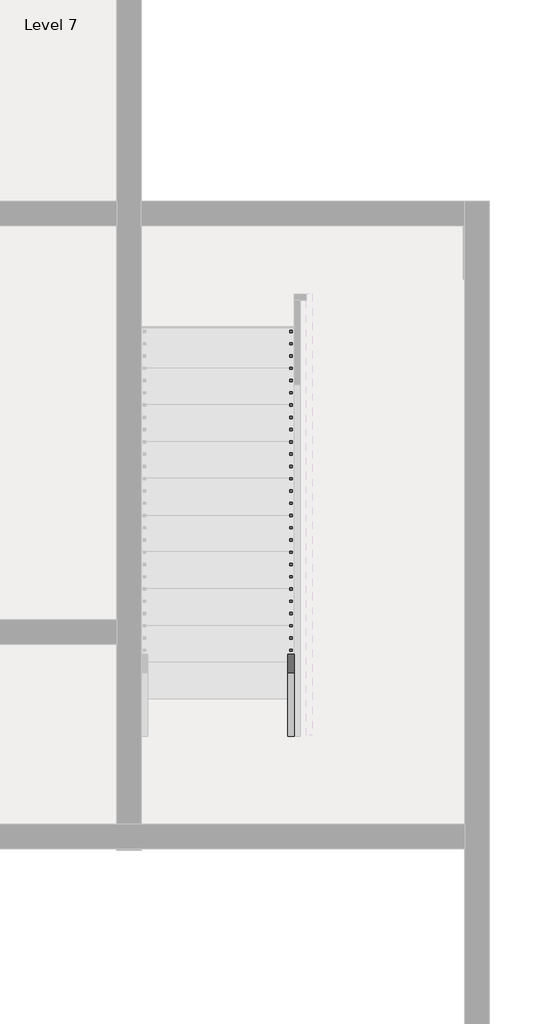
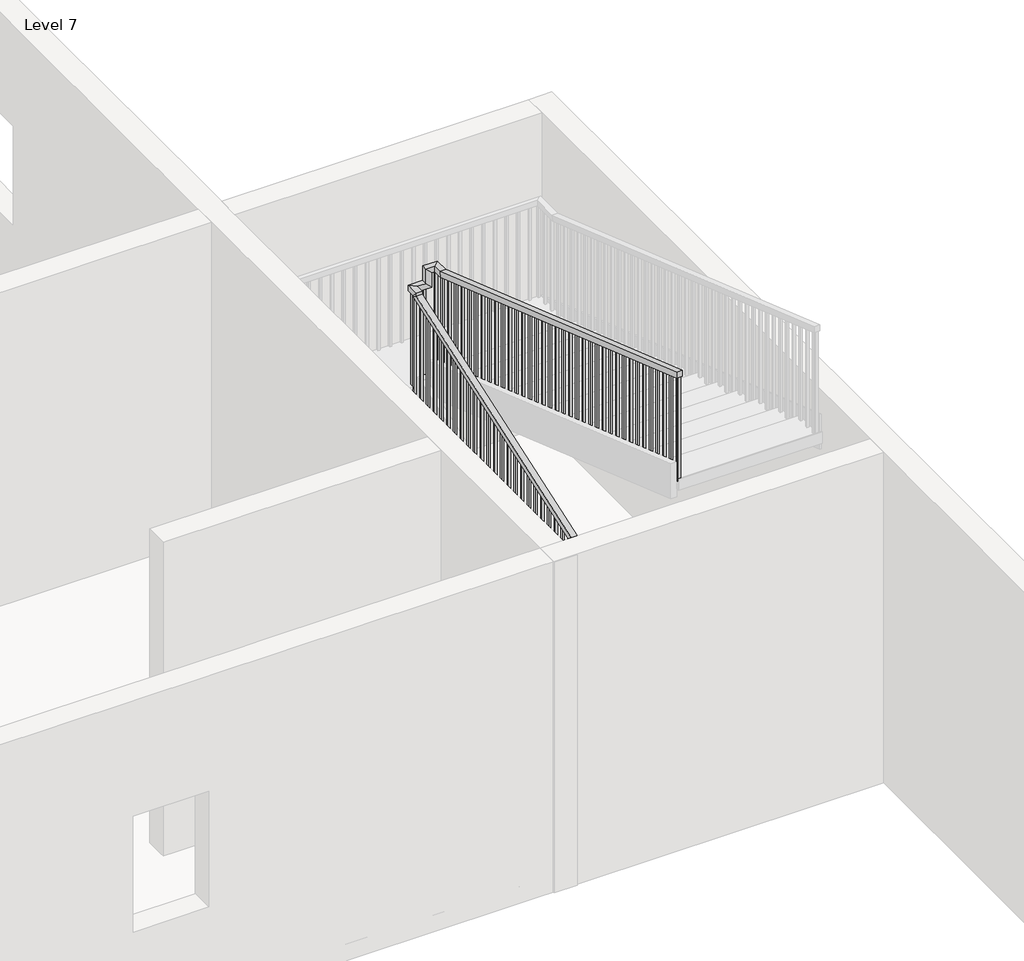
# One storey, part 6 of 14: 1 railing.
"""IFC4 building model written with IfcOpenShell, lengths in millimetres."""

from ifc_helpers import new_model, si_unit, frame, origin, place, context, project, spatial, polyline, outline, extrude, faceted_brep, element, save

model = new_model("IFC4")

# Units and contexts
model_context = context("Model", 3, world=origin())
ifc_project = project(units=[si_unit("LENGTHUNIT", "METRE", prefix="MILLI")], contexts=[model_context])

# Site, building, storey
site = spatial("IfcSite", under=ifc_project)
building = spatial("IfcBuilding", under=site)
storey = spatial("IfcBuildingStorey", under=building, Name="Level 7", Elevation=18288.0)

# Railing
placement = place(None, origin())
element("IfcRailing", 1, ObjectType="Handrail - Rectangular", at=placement, inside=storey, context=model_context, shape_type="SolidModel", body=[
    faceted_brep([(-2644.5381751, -9955.5916506, 19307.9076923), (-2644.5381751, -9955.5916506, 19254.1602476), (-2593.7381751, -9955.5916506, 19254.1602476), (-2593.7381751, -9955.5916506, 19307.9076923), (-2644.5381751, -6367.8416506, 20547.6687908), (-2644.5381751, -6317.0416506, 20511.4754856), (-2593.7381751, -6317.0416506, 20511.4754856), (-2593.7381751, -6367.8416506, 20547.6687908), (-2644.5381751, -6367.8416506, 20574.0), (-2644.5381751, -6317.0416506, 20523.2), (-2593.7381751, -6317.0416506, 20523.2), (-2593.7381751, -6367.8416506, 20574.0), (-2644.5381751, -6240.8416506, 20574.0), (-2644.5381751, -6240.8416506, 20523.2), (-2593.7381751, -6291.6416506, 20523.2), (-2593.7381751, -6291.6416506, 20574.0), (-2517.5381751, -6240.8416506, 20574.0), (-2466.7381751, -6240.8416506, 20523.2), (-2466.7381751, -6291.6416506, 20523.2), (-2517.5381751, -6291.6416506, 20574.0), (-2517.5381751, -6240.8416506, 20705.8846154), (-2466.7381751, -6240.8416506, 20655.0846154), (-2466.7381751, -6291.6416506, 20655.0846154), (-2517.5381751, -6291.6416506, 20705.8846154), (-2390.5381751, -6240.8416506, 20705.8846154), (-2390.5381751, -6240.8416506, 20655.0846154), (-2441.3381751, -6291.6416506, 20655.0846154), (-2441.3381751, -6291.6416506, 20705.8846154), (-2390.5381751, -6367.8416506, 20705.8846154), (-2390.5381751, -6376.3852679, 20655.0846154), (-2441.3381751, -6376.3852679, 20655.0846154), (-2441.3381751, -6367.8416506, 20705.8846154), (-2390.5381751, -9949.2416506, 21945.6), (-2441.3381751, -9949.2416506, 21945.6), (-2441.3381751, -9949.2416506, 21891.842594), (-2390.5381751, -9949.2416506, 21891.842594)], [[[0, 1, 2, 3]], [[1, 0, 4, 5]], [[2, 1, 5, 6]], [[3, 2, 6, 7]], [[0, 3, 7, 4]], [[5, 4, 8, 9]], [[6, 5, 9, 10]], [[7, 6, 10, 11]], [[4, 7, 11, 8]], [[9, 8, 12, 13]], [[10, 9, 13, 14]], [[11, 10, 14, 15]], [[8, 11, 15, 12]], [[13, 12, 16, 17]], [[14, 13, 17, 18]], [[15, 14, 18, 19]], [[12, 15, 19, 16]], [[17, 16, 20, 21]], [[18, 17, 21, 22]], [[19, 18, 22, 23]], [[16, 19, 23, 20]], [[21, 20, 24, 25]], [[22, 21, 25, 26]], [[23, 22, 26, 27]], [[20, 23, 27, 24]], [[25, 24, 28, 29]], [[26, 25, 29, 30]], [[27, 26, 30, 31]], [[24, 27, 31, 28]], [[32, 33, 34, 35]], [[29, 28, 32, 35]], [[30, 29, 35, 34]], [[31, 30, 34, 33]], [[28, 31, 33, 32]]]),
    extrude(outline(polyline([(-9933.3666506, 21886.3474017), (-9914.3166506, 21879.7531709), (-9914.3166506, 20925.6923077), (-9933.3666506, 20925.6923077), (-9933.3666506, 21886.3474017)])), frame((-2425.4631751, 0.0, 0.0), z_axis=(1.0, 0.0, 0.0), x_axis=(0.0, 1.0, 0.0)), (0.0, 0.0, 1.0), 19.05),
    extrude(outline(polyline([(-9831.7666506, 21851.1781709), (-9812.7166506, 21844.5839402), (-9812.7166506, 20925.6923077), (-9831.7666506, 20925.6923077), (-9831.7666506, 21851.1781709)])), frame((-2425.4631751, 0.0, 0.0), z_axis=(1.0, 0.0, 0.0), x_axis=(0.0, 1.0, 0.0)), (0.0, 0.0, 1.0), 19.05),
    extrude(outline(polyline([(-9730.1666506, 21816.0089402), (-9711.1166506, 21809.4147094), (-9711.1166506, 20925.6923077), (-9730.1666506, 20925.6923077), (-9730.1666506, 21816.0089402)])), frame((-2425.4631751, 0.0, 0.0), z_axis=(1.0, 0.0, 0.0), x_axis=(0.0, 1.0, 0.0)), (0.0, 0.0, 1.0), 19.05),
    extrude(outline(polyline([(-9628.5666506, 21780.8397094), (-9609.5166506, 21774.2454786), (-9609.5166506, 20820.1846154), (-9628.5666506, 20820.1846154), (-9628.5666506, 21780.8397094)])), frame((-2425.4631751, 0.0, 0.0), z_axis=(1.0, 0.0, 0.0), x_axis=(0.0, 1.0, 0.0)), (0.0, 0.0, 1.0), 19.05),
    extrude(outline(polyline([(-9526.9666506, 21745.6704786), (-9507.9166506, 21739.0762479), (-9507.9166506, 20820.1846154), (-9526.9666506, 20820.1846154), (-9526.9666506, 21745.6704786)])), frame((-2425.4631751, 0.0, 0.0), z_axis=(1.0, 0.0, 0.0), x_axis=(0.0, 1.0, 0.0)), (0.0, 0.0, 1.0), 19.05),
    extrude(outline(polyline([(-9425.3666506, 21710.5012479), (-9406.3166506, 21703.9070171), (-9406.3166506, 20820.1846154), (-9425.3666506, 20820.1846154), (-9425.3666506, 21710.5012479)])), frame((-2425.4631751, 0.0, 0.0), z_axis=(1.0, 0.0, 0.0), x_axis=(0.0, 1.0, 0.0)), (0.0, 0.0, 1.0), 19.05),
    extrude(outline(polyline([(-9323.7666506, 21675.3320171), (-9304.7166506, 21668.7377863), (-9304.7166506, 20714.6769231), (-9323.7666506, 20714.6769231), (-9323.7666506, 21675.3320171)])), frame((-2425.4631751, 0.0, 0.0), z_axis=(1.0, 0.0, 0.0), x_axis=(0.0, 1.0, 0.0)), (0.0, 0.0, 1.0), 19.05),
    extrude(outline(polyline([(-9222.1666506, 21640.1627863), (-9203.1166506, 21633.5685556), (-9203.1166506, 20714.6769231), (-9222.1666506, 20714.6769231), (-9222.1666506, 21640.1627863)])), frame((-2425.4631751, 0.0, 0.0), z_axis=(1.0, 0.0, 0.0), x_axis=(0.0, 1.0, 0.0)), (0.0, 0.0, 1.0), 19.05),
    extrude(outline(polyline([(-9120.5666506, 21604.9935556), (-9101.5166506, 21598.3993248), (-9101.5166506, 20714.6769231), (-9120.5666506, 20714.6769231), (-9120.5666506, 21604.9935556)])), frame((-2425.4631751, 0.0, 0.0), z_axis=(1.0, 0.0, 0.0), x_axis=(0.0, 1.0, 0.0)), (0.0, 0.0, 1.0), 19.05),
    extrude(outline(polyline([(-9018.9666506, 21569.8243248), (-8999.9166506, 21563.230094), (-8999.9166506, 20609.1692308), (-9018.9666506, 20609.1692308), (-9018.9666506, 21569.8243248)])), frame((-2425.4631751, 0.0, 0.0), z_axis=(1.0, 0.0, 0.0), x_axis=(0.0, 1.0, 0.0)), (0.0, 0.0, 1.0), 19.05),
    extrude(outline(polyline([(-8917.3666506, 21534.655094), (-8898.3166506, 21528.0608632), (-8898.3166506, 20609.1692308), (-8917.3666506, 20609.1692308), (-8917.3666506, 21534.655094)])), frame((-2425.4631751, 0.0, 0.0), z_axis=(1.0, 0.0, 0.0), x_axis=(0.0, 1.0, 0.0)), (0.0, 0.0, 1.0), 19.05),
    extrude(outline(polyline([(-8815.7666506, 21499.4858632), (-8796.7166506, 21492.8916325), (-8796.7166506, 20609.1692308), (-8815.7666506, 20609.1692308), (-8815.7666506, 21499.4858632)])), frame((-2425.4631751, 0.0, 0.0), z_axis=(1.0, 0.0, 0.0), x_axis=(0.0, 1.0, 0.0)), (0.0, 0.0, 1.0), 19.05),
    extrude(outline(polyline([(-8714.1666506, 21464.3166325), (-8695.1166506, 21457.7224017), (-8695.1166506, 20503.6615385), (-8714.1666506, 20503.6615385), (-8714.1666506, 21464.3166325)])), frame((-2425.4631751, 0.0, 0.0), z_axis=(1.0, 0.0, 0.0), x_axis=(0.0, 1.0, 0.0)), (0.0, 0.0, 1.0), 19.05),
    extrude(outline(polyline([(-8612.5666506, 21429.1474017), (-8593.5166506, 21422.5531709), (-8593.5166506, 20503.6615385), (-8612.5666506, 20503.6615385), (-8612.5666506, 21429.1474017)])), frame((-2425.4631751, 0.0, 0.0), z_axis=(1.0, 0.0, 0.0), x_axis=(0.0, 1.0, 0.0)), (0.0, 0.0, 1.0), 19.05),
    extrude(outline(polyline([(-8510.9666506, 21393.9781709), (-8491.9166506, 21387.3839402), (-8491.9166506, 20503.6615385), (-8510.9666506, 20503.6615385), (-8510.9666506, 21393.9781709)])), frame((-2425.4631751, 0.0, 0.0), z_axis=(1.0, 0.0, 0.0), x_axis=(0.0, 1.0, 0.0)), (0.0, 0.0, 1.0), 19.05),
    extrude(outline(polyline([(-8409.3666506, 21358.8089402), (-8390.3166506, 21352.2147094), (-8390.3166506, 20398.1538462), (-8409.3666506, 20398.1538462), (-8409.3666506, 21358.8089402)])), frame((-2425.4631751, 0.0, 0.0), z_axis=(1.0, 0.0, 0.0), x_axis=(0.0, 1.0, 0.0)), (0.0, 0.0, 1.0), 19.05),
    extrude(outline(polyline([(-8307.7666506, 21323.6397094), (-8288.7166506, 21317.0454786), (-8288.7166506, 20398.1538462), (-8307.7666506, 20398.1538462), (-8307.7666506, 21323.6397094)])), frame((-2425.4631751, 0.0, 0.0), z_axis=(1.0, 0.0, 0.0), x_axis=(0.0, 1.0, 0.0)), (0.0, 0.0, 1.0), 19.05),
    extrude(outline(polyline([(-8206.1666506, 21288.4704786), (-8187.1166506, 21281.8762479), (-8187.1166506, 20398.1538462), (-8206.1666506, 20398.1538462), (-8206.1666506, 21288.4704786)])), frame((-2425.4631751, 0.0, 0.0), z_axis=(1.0, 0.0, 0.0), x_axis=(0.0, 1.0, 0.0)), (0.0, 0.0, 1.0), 19.05),
    extrude(outline(polyline([(-8104.5666506, 21253.3012479), (-8085.5166506, 21246.7070171), (-8085.5166506, 20292.6461538), (-8104.5666506, 20292.6461538), (-8104.5666506, 21253.3012479)])), frame((-2425.4631751, 0.0, 0.0), z_axis=(1.0, 0.0, 0.0), x_axis=(0.0, 1.0, 0.0)), (0.0, 0.0, 1.0), 19.05),
    extrude(outline(polyline([(-8002.9666506, 21218.1320171), (-7983.9166506, 21211.5377863), (-7983.9166506, 20292.6461538), (-8002.9666506, 20292.6461538), (-8002.9666506, 21218.1320171)])), frame((-2425.4631751, 0.0, 0.0), z_axis=(1.0, 0.0, 0.0), x_axis=(0.0, 1.0, 0.0)), (0.0, 0.0, 1.0), 19.05),
    extrude(outline(polyline([(-7901.3666506, 21182.9627863), (-7882.3166506, 21176.3685556), (-7882.3166506, 20292.6461538), (-7901.3666506, 20292.6461538), (-7901.3666506, 21182.9627863)])), frame((-2425.4631751, 0.0, 0.0), z_axis=(1.0, 0.0, 0.0), x_axis=(0.0, 1.0, 0.0)), (0.0, 0.0, 1.0), 19.05),
    extrude(outline(polyline([(-7799.7666506, 21147.7935556), (-7780.7166506, 21141.1993248), (-7780.7166506, 20187.1384615), (-7799.7666506, 20187.1384615), (-7799.7666506, 21147.7935556)])), frame((-2425.4631751, 0.0, 0.0), z_axis=(1.0, 0.0, 0.0), x_axis=(0.0, 1.0, 0.0)), (0.0, 0.0, 1.0), 19.05),
    extrude(outline(polyline([(-7698.1666506, 21112.6243248), (-7679.1166506, 21106.030094), (-7679.1166506, 20187.1384615), (-7698.1666506, 20187.1384615), (-7698.1666506, 21112.6243248)])), frame((-2425.4631751, 0.0, 0.0), z_axis=(1.0, 0.0, 0.0), x_axis=(0.0, 1.0, 0.0)), (0.0, 0.0, 1.0), 19.05),
    extrude(outline(polyline([(-7596.5666506, 21077.455094), (-7577.5166506, 21070.8608632), (-7577.5166506, 20187.1384615), (-7596.5666506, 20187.1384615), (-7596.5666506, 21077.455094)])), frame((-2425.4631751, 0.0, 0.0), z_axis=(1.0, 0.0, 0.0), x_axis=(0.0, 1.0, 0.0)), (0.0, 0.0, 1.0), 19.05),
    extrude(outline(polyline([(-7494.9666506, 21042.2858632), (-7475.9166506, 21035.6916325), (-7475.9166506, 20081.6307692), (-7494.9666506, 20081.6307692), (-7494.9666506, 21042.2858632)])), frame((-2425.4631751, 0.0, 0.0), z_axis=(1.0, 0.0, 0.0), x_axis=(0.0, 1.0, 0.0)), (0.0, 0.0, 1.0), 19.05),
    extrude(outline(polyline([(-7393.3666506, 21007.1166325), (-7374.3166506, 21000.5224017), (-7374.3166506, 20081.6307692), (-7393.3666506, 20081.6307692), (-7393.3666506, 21007.1166325)])), frame((-2425.4631751, 0.0, 0.0), z_axis=(1.0, 0.0, 0.0), x_axis=(0.0, 1.0, 0.0)), (0.0, 0.0, 1.0), 19.05),
    extrude(outline(polyline([(-7291.7666506, 20971.9474017), (-7272.7166506, 20965.3531709), (-7272.7166506, 20081.6307692), (-7291.7666506, 20081.6307692), (-7291.7666506, 20971.9474017)])), frame((-2425.4631751, 0.0, 0.0), z_axis=(1.0, 0.0, 0.0), x_axis=(0.0, 1.0, 0.0)), (0.0, 0.0, 1.0), 19.05),
    extrude(outline(polyline([(-7190.1666506, 20936.7781709), (-7171.1166506, 20930.1839402), (-7171.1166506, 19976.1230769), (-7190.1666506, 19976.1230769), (-7190.1666506, 20936.7781709)])), frame((-2425.4631751, 0.0, 0.0), z_axis=(1.0, 0.0, 0.0), x_axis=(0.0, 1.0, 0.0)), (0.0, 0.0, 1.0), 19.05),
    extrude(outline(polyline([(-7088.5666506, 20901.6089402), (-7069.5166506, 20895.0147094), (-7069.5166506, 19976.1230769), (-7088.5666506, 19976.1230769), (-7088.5666506, 20901.6089402)])), frame((-2425.4631751, 0.0, 0.0), z_axis=(1.0, 0.0, 0.0), x_axis=(0.0, 1.0, 0.0)), (0.0, 0.0, 1.0), 19.05),
    extrude(outline(polyline([(-6986.9666506, 20866.4397094), (-6967.9166506, 20859.8454786), (-6967.9166506, 19976.1230769), (-6986.9666506, 19976.1230769), (-6986.9666506, 20866.4397094)])), frame((-2425.4631751, 0.0, 0.0), z_axis=(1.0, 0.0, 0.0), x_axis=(0.0, 1.0, 0.0)), (0.0, 0.0, 1.0), 19.05),
    extrude(outline(polyline([(-6885.3666506, 20831.2704786), (-6866.3166506, 20824.6762479), (-6866.3166506, 19870.6153846), (-6885.3666506, 19870.6153846), (-6885.3666506, 20831.2704786)])), frame((-2425.4631751, 0.0, 0.0), z_axis=(1.0, 0.0, 0.0), x_axis=(0.0, 1.0, 0.0)), (0.0, 0.0, 1.0), 19.05),
    extrude(outline(polyline([(-6783.7666506, 20796.1012479), (-6764.7166506, 20789.5070171), (-6764.7166506, 19870.6153846), (-6783.7666506, 19870.6153846), (-6783.7666506, 20796.1012479)])), frame((-2425.4631751, 0.0, 0.0), z_axis=(1.0, 0.0, 0.0), x_axis=(0.0, 1.0, 0.0)), (0.0, 0.0, 1.0), 19.05),
    extrude(outline(polyline([(-6682.1666506, 20760.9320171), (-6663.1166506, 20754.3377863), (-6663.1166506, 19870.6153846), (-6682.1666506, 19870.6153846), (-6682.1666506, 20760.9320171)])), frame((-2425.4631751, 0.0, 0.0), z_axis=(1.0, 0.0, 0.0), x_axis=(0.0, 1.0, 0.0)), (0.0, 0.0, 1.0), 19.05),
    extrude(outline(polyline([(-6580.5666506, 20725.7627863), (-6561.5166506, 20719.1685556), (-6561.5166506, 19765.1076923), (-6580.5666506, 19765.1076923), (-6580.5666506, 20725.7627863)])), frame((-2425.4631751, 0.0, 0.0), z_axis=(1.0, 0.0, 0.0), x_axis=(0.0, 1.0, 0.0)), (0.0, 0.0, 1.0), 19.05),
    extrude(outline(polyline([(-6478.9666506, 20690.5935556), (-6459.9166506, 20683.9993248), (-6459.9166506, 19765.1076923), (-6478.9666506, 19765.1076923), (-6478.9666506, 20690.5935556)])), frame((-2425.4631751, 0.0, 0.0), z_axis=(1.0, 0.0, 0.0), x_axis=(0.0, 1.0, 0.0)), (0.0, 0.0, 1.0), 19.05),
    extrude(outline(polyline([(-6377.3666506, 20655.4243248), (-6358.3166506, 20648.830094), (-6358.3166506, 19765.1076923), (-6377.3666506, 19765.1076923), (-6377.3666506, 20655.4243248)])), frame((-2425.4631751, 0.0, 0.0), z_axis=(1.0, 0.0, 0.0), x_axis=(0.0, 1.0, 0.0)), (0.0, 0.0, 1.0), 19.05),
    extrude(outline(polyline([(-2527.0631751, -6275.7666506), (-2527.0631751, -6256.7166506), (-2508.0131751, -6256.7166506), (-2508.0131751, -6275.7666506), (-2527.0631751, -6275.7666506)])), frame((0.0, 0.0, 19659.6), z_axis=(0.0, 0.0, 1.0), x_axis=(1.0, 0.0, 0.0)), (0.0, 0.0, 1.0), 863.6),
    extrude(outline(polyline([(-2609.6131751, -6307.5166506), (-2628.6631751, -6307.5166506), (-2628.6631751, -6288.4666506), (-2609.6131751, -6288.4666506), (-2609.6131751, -6307.5166506)])), frame((0.0, 0.0, 19554.0923077), z_axis=(0.0, 0.0, 1.0), x_axis=(1.0, 0.0, 0.0)), (0.0, 0.0, 1.0), 969.1076923),
    extrude(outline(polyline([(-6409.1166506, 20479.6586078), (-6390.0666506, 20486.2414101), (-6390.0666506, 19554.0923077), (-6409.1166506, 19554.0923077), (-6409.1166506, 20479.6586078)])), frame((-2628.6631751, 0.0, 0.0), z_axis=(1.0, 0.0, 0.0), x_axis=(0.0, 1.0, 0.0)), (0.0, 0.0, 1.0), 19.05),
    extrude(outline(polyline([(-6510.7166506, 20444.5503289), (-6491.6666506, 20451.1331312), (-6491.6666506, 19554.0923077), (-6510.7166506, 19554.0923077), (-6510.7166506, 20444.5503289)])), frame((-2628.6631751, 0.0, 0.0), z_axis=(1.0, 0.0, 0.0), x_axis=(0.0, 1.0, 0.0)), (0.0, 0.0, 1.0), 19.05),
    extrude(outline(polyline([(-6612.3166506, 20409.44205), (-6593.2666506, 20416.0248523), (-6593.2666506, 19448.5846154), (-6612.3166506, 19448.5846154), (-6612.3166506, 20409.44205)])), frame((-2628.6631751, 0.0, 0.0), z_axis=(1.0, 0.0, 0.0), x_axis=(0.0, 1.0, 0.0)), (0.0, 0.0, 1.0), 19.05),
    extrude(outline(polyline([(-6713.9166506, 20374.3337711), (-6694.8666506, 20380.9165734), (-6694.8666506, 19448.5846154), (-6713.9166506, 19448.5846154), (-6713.9166506, 20374.3337711)])), frame((-2628.6631751, 0.0, 0.0), z_axis=(1.0, 0.0, 0.0), x_axis=(0.0, 1.0, 0.0)), (0.0, 0.0, 1.0), 19.05),
    extrude(outline(polyline([(-6815.5166506, 20339.2254922), (-6796.4666506, 20345.8082945), (-6796.4666506, 19448.5846154), (-6815.5166506, 19448.5846154), (-6815.5166506, 20339.2254922)])), frame((-2628.6631751, 0.0, 0.0), z_axis=(1.0, 0.0, 0.0), x_axis=(0.0, 1.0, 0.0)), (0.0, 0.0, 1.0), 19.05),
    extrude(outline(polyline([(-6917.1166506, 20304.1172133), (-6898.0666506, 20310.7000156), (-6898.0666506, 19343.0769231), (-6917.1166506, 19343.0769231), (-6917.1166506, 20304.1172133)])), frame((-2628.6631751, 0.0, 0.0), z_axis=(1.0, 0.0, 0.0), x_axis=(0.0, 1.0, 0.0)), (0.0, 0.0, 1.0), 19.05),
    extrude(outline(polyline([(-7018.7166506, 20269.0089344), (-6999.6666506, 20275.5917367), (-6999.6666506, 19343.0769231), (-7018.7166506, 19343.0769231), (-7018.7166506, 20269.0089344)])), frame((-2628.6631751, 0.0, 0.0), z_axis=(1.0, 0.0, 0.0), x_axis=(0.0, 1.0, 0.0)), (0.0, 0.0, 1.0), 19.05),
    extrude(outline(polyline([(-7120.3166506, 20233.9006556), (-7101.2666506, 20240.4834578), (-7101.2666506, 19343.0769231), (-7120.3166506, 19343.0769231), (-7120.3166506, 20233.9006556)])), frame((-2628.6631751, 0.0, 0.0), z_axis=(1.0, 0.0, 0.0), x_axis=(0.0, 1.0, 0.0)), (0.0, 0.0, 1.0), 19.05),
    extrude(outline(polyline([(-7221.9166506, 20198.7923767), (-7202.8666506, 20205.375179), (-7202.8666506, 19237.5692308), (-7221.9166506, 19237.5692308), (-7221.9166506, 20198.7923767)])), frame((-2628.6631751, 0.0, 0.0), z_axis=(1.0, 0.0, 0.0), x_axis=(0.0, 1.0, 0.0)), (0.0, 0.0, 1.0), 19.05),
    extrude(outline(polyline([(-7323.5166506, 20163.6840978), (-7304.4666506, 20170.2669001), (-7304.4666506, 19237.5692308), (-7323.5166506, 19237.5692308), (-7323.5166506, 20163.6840978)])), frame((-2628.6631751, 0.0, 0.0), z_axis=(1.0, 0.0, 0.0), x_axis=(0.0, 1.0, 0.0)), (0.0, 0.0, 1.0), 19.05),
    extrude(outline(polyline([(-7425.1166506, 20128.5758189), (-7406.0666506, 20135.1586212), (-7406.0666506, 19237.5692308), (-7425.1166506, 19237.5692308), (-7425.1166506, 20128.5758189)])), frame((-2628.6631751, 0.0, 0.0), z_axis=(1.0, 0.0, 0.0), x_axis=(0.0, 1.0, 0.0)), (0.0, 0.0, 1.0), 19.05),
    extrude(outline(polyline([(-7526.7166506, 20093.46754), (-7507.6666506, 20100.0503423), (-7507.6666506, 19132.0615385), (-7526.7166506, 19132.0615385), (-7526.7166506, 20093.46754)])), frame((-2628.6631751, 0.0, 0.0), z_axis=(1.0, 0.0, 0.0), x_axis=(0.0, 1.0, 0.0)), (0.0, 0.0, 1.0), 19.05),
    extrude(outline(polyline([(-7628.3166506, 20058.3592611), (-7609.2666506, 20064.9420634), (-7609.2666506, 19132.0615385), (-7628.3166506, 19132.0615385), (-7628.3166506, 20058.3592611)])), frame((-2628.6631751, 0.0, 0.0), z_axis=(1.0, 0.0, 0.0), x_axis=(0.0, 1.0, 0.0)), (0.0, 0.0, 1.0), 19.05),
    extrude(outline(polyline([(-7729.9166506, 20023.2509822), (-7710.8666506, 20029.8337845), (-7710.8666506, 19132.0615385), (-7729.9166506, 19132.0615385), (-7729.9166506, 20023.2509822)])), frame((-2628.6631751, 0.0, 0.0), z_axis=(1.0, 0.0, 0.0), x_axis=(0.0, 1.0, 0.0)), (0.0, 0.0, 1.0), 19.05),
    extrude(outline(polyline([(-7831.5166506, 19988.1427033), (-7812.4666506, 19994.7255056), (-7812.4666506, 19026.5538462), (-7831.5166506, 19026.5538462), (-7831.5166506, 19988.1427033)])), frame((-2628.6631751, 0.0, 0.0), z_axis=(1.0, 0.0, 0.0), x_axis=(0.0, 1.0, 0.0)), (0.0, 0.0, 1.0), 19.05),
    extrude(outline(polyline([(-7933.1166506, 19953.0344244), (-7914.0666506, 19959.6172267), (-7914.0666506, 19026.5538462), (-7933.1166506, 19026.5538462), (-7933.1166506, 19953.0344244)])), frame((-2628.6631751, 0.0, 0.0), z_axis=(1.0, 0.0, 0.0), x_axis=(0.0, 1.0, 0.0)), (0.0, 0.0, 1.0), 19.05),
    extrude(outline(polyline([(-8034.7166506, 19917.9261455), (-8015.6666506, 19924.5089478), (-8015.6666506, 19026.5538462), (-8034.7166506, 19026.5538462), (-8034.7166506, 19917.9261455)])), frame((-2628.6631751, 0.0, 0.0), z_axis=(1.0, 0.0, 0.0), x_axis=(0.0, 1.0, 0.0)), (0.0, 0.0, 1.0), 19.05),
    extrude(outline(polyline([(-8136.3166506, 19882.8178666), (-8117.2666506, 19889.4006689), (-8117.2666506, 18921.0461538), (-8136.3166506, 18921.0461538), (-8136.3166506, 19882.8178666)])), frame((-2628.6631751, 0.0, 0.0), z_axis=(1.0, 0.0, 0.0), x_axis=(0.0, 1.0, 0.0)), (0.0, 0.0, 1.0), 19.05),
    extrude(outline(polyline([(-8237.9166506, 19847.7095877), (-8218.8666506, 19854.29239), (-8218.8666506, 18921.0461538), (-8237.9166506, 18921.0461538), (-8237.9166506, 19847.7095877)])), frame((-2628.6631751, 0.0, 0.0), z_axis=(1.0, 0.0, 0.0), x_axis=(0.0, 1.0, 0.0)), (0.0, 0.0, 1.0), 19.05),
    extrude(outline(polyline([(-8339.5166506, 19812.6013088), (-8320.4666506, 19819.1841111), (-8320.4666506, 18921.0461538), (-8339.5166506, 18921.0461538), (-8339.5166506, 19812.6013088)])), frame((-2628.6631751, 0.0, 0.0), z_axis=(1.0, 0.0, 0.0), x_axis=(0.0, 1.0, 0.0)), (0.0, 0.0, 1.0), 19.05),
    extrude(outline(polyline([(-8441.1166506, 19777.4930299), (-8422.0666506, 19784.0758322), (-8422.0666506, 18815.5384615), (-8441.1166506, 18815.5384615), (-8441.1166506, 19777.4930299)])), frame((-2628.6631751, 0.0, 0.0), z_axis=(1.0, 0.0, 0.0), x_axis=(0.0, 1.0, 0.0)), (0.0, 0.0, 1.0), 19.05),
    extrude(outline(polyline([(-8542.7166506, 19742.384751), (-8523.6666506, 19748.9675533), (-8523.6666506, 18815.5384615), (-8542.7166506, 18815.5384615), (-8542.7166506, 19742.384751)])), frame((-2628.6631751, 0.0, 0.0), z_axis=(1.0, 0.0, 0.0), x_axis=(0.0, 1.0, 0.0)), (0.0, 0.0, 1.0), 19.05),
    extrude(outline(polyline([(-8644.3166506, 19707.2764721), (-8625.2666506, 19713.8592744), (-8625.2666506, 18815.5384615), (-8644.3166506, 18815.5384615), (-8644.3166506, 19707.2764721)])), frame((-2628.6631751, 0.0, 0.0), z_axis=(1.0, 0.0, 0.0), x_axis=(0.0, 1.0, 0.0)), (0.0, 0.0, 1.0), 19.05),
    extrude(outline(polyline([(-8745.9166506, 19672.1681932), (-8726.8666506, 19678.7509955), (-8726.8666506, 18710.0307692), (-8745.9166506, 18710.0307692), (-8745.9166506, 19672.1681932)])), frame((-2628.6631751, 0.0, 0.0), z_axis=(1.0, 0.0, 0.0), x_axis=(0.0, 1.0, 0.0)), (0.0, 0.0, 1.0), 19.05),
    extrude(outline(polyline([(-8847.5166506, 19637.0599143), (-8828.4666506, 19643.6427166), (-8828.4666506, 18710.0307692), (-8847.5166506, 18710.0307692), (-8847.5166506, 19637.0599143)])), frame((-2628.6631751, 0.0, 0.0), z_axis=(1.0, 0.0, 0.0), x_axis=(0.0, 1.0, 0.0)), (0.0, 0.0, 1.0), 19.05),
    extrude(outline(polyline([(-8949.1166506, 19601.9516354), (-8930.0666506, 19608.5344377), (-8930.0666506, 18710.0307692), (-8949.1166506, 18710.0307692), (-8949.1166506, 19601.9516354)])), frame((-2628.6631751, 0.0, 0.0), z_axis=(1.0, 0.0, 0.0), x_axis=(0.0, 1.0, 0.0)), (0.0, 0.0, 1.0), 19.05),
    extrude(outline(polyline([(-9050.7166506, 19566.8433565), (-9031.6666506, 19573.4261588), (-9031.6666506, 18604.5230769), (-9050.7166506, 18604.5230769), (-9050.7166506, 19566.8433565)])), frame((-2628.6631751, 0.0, 0.0), z_axis=(1.0, 0.0, 0.0), x_axis=(0.0, 1.0, 0.0)), (0.0, 0.0, 1.0), 19.05),
    extrude(outline(polyline([(-9152.3166506, 19531.7350776), (-9133.2666506, 19538.3178799), (-9133.2666506, 18604.5230769), (-9152.3166506, 18604.5230769), (-9152.3166506, 19531.7350776)])), frame((-2628.6631751, 0.0, 0.0), z_axis=(1.0, 0.0, 0.0), x_axis=(0.0, 1.0, 0.0)), (0.0, 0.0, 1.0), 19.05),
    extrude(outline(polyline([(-9253.9166506, 19496.6267987), (-9234.8666506, 19503.209601), (-9234.8666506, 18604.5230769), (-9253.9166506, 18604.5230769), (-9253.9166506, 19496.6267987)])), frame((-2628.6631751, 0.0, 0.0), z_axis=(1.0, 0.0, 0.0), x_axis=(0.0, 1.0, 0.0)), (0.0, 0.0, 1.0), 19.05),
    extrude(outline(polyline([(-9355.5166506, 19461.5185198), (-9336.4666506, 19468.1013221), (-9336.4666506, 18499.0153846), (-9355.5166506, 18499.0153846), (-9355.5166506, 19461.5185198)])), frame((-2628.6631751, 0.0, 0.0), z_axis=(1.0, 0.0, 0.0), x_axis=(0.0, 1.0, 0.0)), (0.0, 0.0, 1.0), 19.05),
    extrude(outline(polyline([(-9457.1166506, 19426.4102409), (-9438.0666506, 19432.9930432), (-9438.0666506, 18499.0153846), (-9457.1166506, 18499.0153846), (-9457.1166506, 19426.4102409)])), frame((-2628.6631751, 0.0, 0.0), z_axis=(1.0, 0.0, 0.0), x_axis=(0.0, 1.0, 0.0)), (0.0, 0.0, 1.0), 19.05),
    extrude(outline(polyline([(-9558.7166506, 19391.301962), (-9539.6666506, 19397.8847643), (-9539.6666506, 18499.0153846), (-9558.7166506, 18499.0153846), (-9558.7166506, 19391.301962)])), frame((-2628.6631751, 0.0, 0.0), z_axis=(1.0, 0.0, 0.0), x_axis=(0.0, 1.0, 0.0)), (0.0, 0.0, 1.0), 19.05),
    extrude(outline(polyline([(-9660.3166506, 19356.1936831), (-9641.2666506, 19362.7764854), (-9641.2666506, 18393.5076923), (-9660.3166506, 18393.5076923), (-9660.3166506, 19356.1936831)])), frame((-2628.6631751, 0.0, 0.0), z_axis=(1.0, 0.0, 0.0), x_axis=(0.0, 1.0, 0.0)), (0.0, 0.0, 1.0), 19.05),
    extrude(outline(polyline([(-9761.9166506, 19321.0854043), (-9742.8666506, 19327.6682065), (-9742.8666506, 18393.5076923), (-9761.9166506, 18393.5076923), (-9761.9166506, 19321.0854043)])), frame((-2628.6631751, 0.0, 0.0), z_axis=(1.0, 0.0, 0.0), x_axis=(0.0, 1.0, 0.0)), (0.0, 0.0, 1.0), 19.05),
    extrude(outline(polyline([(-9863.5166506, 19285.9771254), (-9844.4666506, 19292.5599277), (-9844.4666506, 18393.5076923), (-9863.5166506, 18393.5076923), (-9863.5166506, 19285.9771254)])), frame((-2628.6631751, 0.0, 0.0), z_axis=(1.0, 0.0, 0.0), x_axis=(0.0, 1.0, 0.0)), (0.0, 0.0, 1.0), 19.05),
    extrude(outline(polyline([(-2425.4631751, -6275.7666506), (-2425.4631751, -6256.7166506), (-2406.4131751, -6256.7166506), (-2406.4131751, -6275.7666506), (-2425.4631751, -6275.7666506)])), frame((0.0, 0.0, 19659.6), z_axis=(0.0, 0.0, 1.0), x_axis=(1.0, 0.0, 0.0)), (0.0, 0.0, 1.0), 995.4846154),
    extrude(outline(polyline([(-2609.6131751, -6275.7666506), (-2628.6631751, -6275.7666506), (-2628.6631751, -6256.7166506), (-2609.6131751, -6256.7166506), (-2609.6131751, -6275.7666506)])), frame((0.0, 0.0, 19659.6), z_axis=(0.0, 0.0, 1.0), x_axis=(1.0, 0.0, 0.0)), (0.0, 0.0, 1.0), 863.6),
    extrude(outline(polyline([(-9949.2416506, 21891.842594), (-9930.1916506, 21885.2483632), (-9930.1916506, 20925.6923077), (-9949.2416506, 20925.6923077), (-9949.2416506, 21891.842594)])), frame((-2425.4631751, 0.0, 0.0), z_axis=(1.0, 0.0, 0.0), x_axis=(0.0, 1.0, 0.0)), (0.0, 0.0, 1.0), 19.05),
    extrude(outline(polyline([(-9955.5916506, 19254.1602476), (-9936.5416506, 19260.7430499), (-9936.5416506, 18393.5076923), (-9955.5916506, 18393.5076923), (-9955.5916506, 19254.1602476)])), frame((-2628.6631751, 0.0, 0.0), z_axis=(1.0, 0.0, 0.0), x_axis=(0.0, 1.0, 0.0)), (0.0, 0.0, 1.0), 19.05),
])

save(model, "model.ifc")

# Revit data of these elements
# Type "Handrail - Rectangular"
#   Assembly Code = "C2010400"
#   built-in parameter 1008612 = 0.0416667 (stored number, unit not read)
#   built-in parameter 1008611 = 0.0416667 (stored number, unit not read)
#   built-in parameter 1008609 = 0.333333 (stored number, unit not read)
#   built-in parameter 1008604 = 0.166667 (stored number, unit not read)
#   built-in parameter 1008603 = 0.166667 (stored number, unit not read)
#   Railing Height = 3' - 0"
#   built-in parameter 1008630 = 2
#   built-in parameter 1008610 = 2
#   built-in parameter 1008618 = Baluster - Square : 3/4"
# Element 1 (IfcRailing, "Handrail - Rectangular")
#   Phase Created = New Construction
